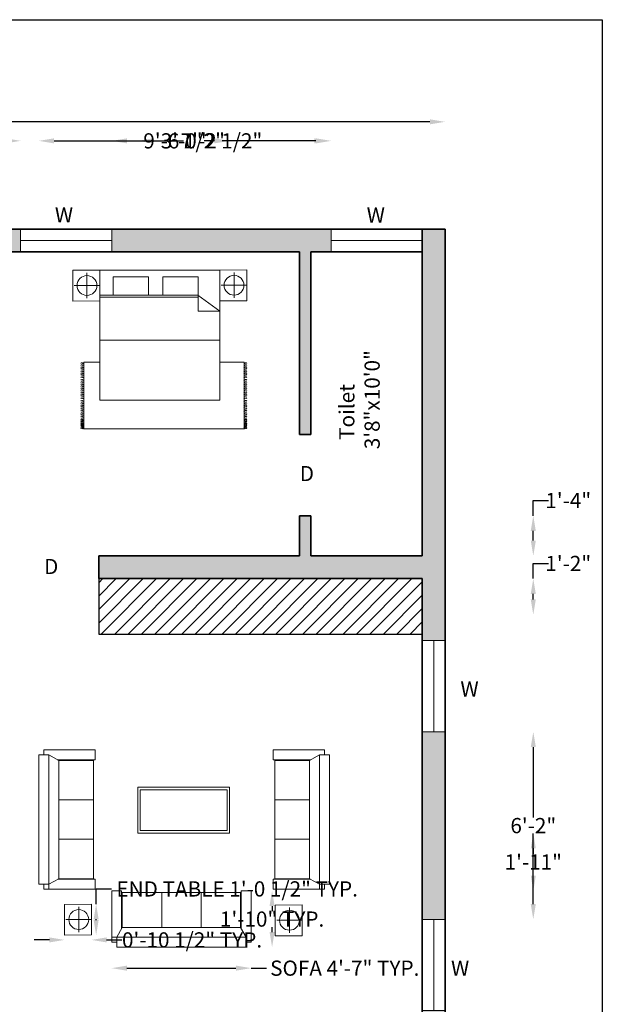
# Model space of a CAD drawing. Units: inches. Extents: x 1054 to 1577, y 4847 to 5610.
# Tile 5 of 5: x 1347 to 1577, y 5221 to 5610. Entities that reach past the tile are written whole.
import ezdxf

# ---------------------------------------------------------------- set-up
doc = ezdxf.new("R2010")
doc.units = ezdxf.units.IN
doc.header["$MEASUREMENT"] = 0
for name, color, linetype, lineweight in [('A-ANNO-DIMS', 2, 'Continuous', 18), ('A-ANNO-TEXT', 7, 'Continuous', 18), ('A-ANNO-TTLB', 7, 'Continuous', 25), ('A-AREA-IDEN', 7, 'Continuous', 18), ('A-FLOR-CASE', 7, 'Continuous', 25), ('A-FLOR-CASE-PATT', 252, 'Continuous', 13), ('A-GLAZ', 4, 'Continuous', 18), ('A-WALL', 7, 'Continuous', 35)]:
    doc.layers.add(name, color=color, linetype=linetype, lineweight=lineweight)
doc.layers.add('A-FURN', color=40, linetype='Continuous', lineweight=18, true_color=0xf8d731)
doc.layers.add('A-WALL-PATT', color=240, linetype='Continuous', lineweight=13, true_color=0xed1f24)
doc.styles.get("Standard").update_dxf_attribs({"font": 'arial.ttf'})
doc.dimstyles.get("Standard").update_dxf_attribs({"dimtxt": 6, "dimasz": 6, "dimexe": 0.18, "dimexo": 0.0625, "dimgap": 0.09, "dimtad": 0, "dimtih": 1, "dimtoh": 1, "dimdec": 1, "dimzin": 0, "dimdsep": 46, "dimlunit": 3, "dimtxsty": 'Standard', "dimcen": 0.09, "dimse1": 1, "dimse2": 1, "dimadec": 0, "dimazin": 0, "dimtfac": 1, "dimtdec": 1, "dimtofl": 0, "dimtmove": 0, "dimatfit": 3, "dimfxl": 1, "dimtolj": 1, "dimtzin": 0, "dimarcsym": 0})

# ---------------------------------------------------------------- blocks, each defined once
blk = doc.blocks.new('*D4')
at = {"layer": 'A-ANNO-DIMS', "color": 0, "lineweight": -2, "transparency": 16777216}
for p, q in [((1136.77, 5569.79), (1309.14, 5569.79)), ((1509.27, 5569.79), (1336.91, 5569.79))]:
    blk.add_line(p, q, dxfattribs=at)
at = {"layer": 'A-ANNO-DIMS', "color": 0, "transparency": 16777216}
for points in [[(1136.77, 5570.79), (1136.77, 5568.79), (1130.77, 5569.79)], [(1509.27, 5570.79), (1509.27, 5568.79), (1515.27, 5569.79)]]:
    blk.add_solid(points, dxfattribs=at)
at = {"layer": 'Defpoints', "color": 0, "transparency": 16777216}
for p in [(1515.27, 5569.79), (1130.77, 5527.48), (1515.27, 5527.48)]:
    blk.add_point(p, dxfattribs=at)
at = {"layer": 'A-ANNO-DIMS', "color": 0, "transparency": 16777216, "insert": (1323.02, 5569.79), "char_height": 6, "attachment_point": 5}
blk.add_mtext('\\A1;32\'-0.5"', dxfattribs=at)
blk = doc.blocks.new('WINDOW-36IN')
for p, q in [((0, 9), (0, 0)), ((36, 9), (0, 9)), ((36, 0), (36, 9)), ((36, 4.5), (0, 4.5)), ((0, 0), (36, 0))]:
    blk.add_line(p, q)
blk = doc.blocks.new('BED-DOUBLE-WITH-TABLES')
for p, q in [((5.6, 61.62), (5.6, 51.56)), ((63.65, 61.72), (63.65, 51.66)), ((10.63, 56.59), (0.57, 56.59)), ((68.68, 56.69), (58.62, 56.69)), ((49.39, 52.82), (10.63, 52.82)), ((49.44, 52), (10.63, 52)), ((49.39, 52.82), (58, 46.47)), ((49.44, 52.82), (49.44, 46.47)), ((49.44, 46.47), (58, 46.47)), ((58.05, 34.96), (10.63, 34.96)), ((4.35, 0), (4.35, 26.37)), ((4.35, 26.37), (10.65, 26.37)), ((58.05, 26.37), (67.59, 26.37)), ((67.59, 26.37), (67.59, 0)), ((67.59, 0), (4.35, 0))]:
    blk.add_line(p, q)
for points in [[(0, 50.39), (10.63, 50.5), (10.63, 62.68), (0, 62.58)], [(58.05, 62.68), (58.05, 11.37), (10.63, 11.37), (10.63, 62.68)], [(58.05, 50.5), (68.68, 50.6), (68.68, 62.78), (58.05, 62.68)], [(29.88, 59.98), (29.88, 52.82), (15.98, 52.82), (15.98, 59.98)], [(49.44, 59.98), (49.44, 52.82), (35.55, 52.82), (35.55, 59.98)]]:
    blk.add_lwpolyline(points, close=True)
for centre in [(5.6, 56.59), (63.65, 56.69)]:
    blk.add_circle(centre, 3.92)
for points, knots in [([(3.23, 25.84), (3.32, 25.96), (3.52, 26.2), (3.86, 25.96), (4.14, 25.78), (4.29, 25.89), (4.35, 25.94)], [0, 0, 0, 0, 0.400747, 0.791423, 1.067667, 1.29709, 1.29709, 1.29709, 1.29709]), ([(3.23, 25.06), (3.32, 25.18), (3.52, 25.42), (3.86, 25.18), (4.14, 25.01), (4.29, 25.11), (4.35, 25.16)], [0, 0, 0, 0, 0.400747, 0.791423, 1.067667, 1.29709, 1.29709, 1.29709, 1.29709]), ([(3.23, 24.24), (3.32, 24.36), (3.52, 24.6), (3.86, 24.36), (4.14, 24.19), (4.29, 24.3), (4.35, 24.34)], [0, 0, 0, 0, 0.400747, 0.791423, 1.067667, 1.29709, 1.29709, 1.29709, 1.29709]), ([(3.23, 23.51), (3.32, 23.63), (3.52, 23.87), (3.86, 23.63), (4.14, 23.46), (4.29, 23.57), (4.35, 23.62)], [0, 0, 0, 0, 0.400747, 0.791423, 1.067667, 1.29709, 1.29709, 1.29709, 1.29709]), ([(68.71, 25.84), (68.61, 25.96), (68.42, 26.2), (68.08, 25.96), (67.8, 25.78), (67.65, 25.89), (67.58, 25.94)], [0, 0, 0, 0, 0.400747, 0.791423, 1.067667, 1.29709, 1.29709, 1.29709, 1.29709]), ([(68.71, 25.06), (68.61, 25.18), (68.42, 25.42), (68.08, 25.18), (67.8, 25.01), (67.65, 25.11), (67.58, 25.16)], [0, 0, 0, 0, 0.400747, 0.791423, 1.067667, 1.29709, 1.29709, 1.29709, 1.29709]), ([(68.71, 24.24), (68.61, 24.36), (68.42, 24.6), (68.08, 24.36), (67.8, 24.19), (67.65, 24.3), (67.58, 24.34)], [0, 0, 0, 0, 0.400747, 0.791423, 1.067667, 1.29709, 1.29709, 1.29709, 1.29709]), ([(68.71, 23.51), (68.61, 23.63), (68.42, 23.87), (68.08, 23.63), (67.8, 23.46), (67.65, 23.57), (67.58, 23.62)], [0, 0, 0, 0, 0.400747, 0.791423, 1.067667, 1.29709, 1.29709, 1.29709, 1.29709]), ([(3.23, 22.63), (3.32, 22.75), (3.52, 22.99), (3.86, 22.75), (4.14, 22.58), (4.29, 22.69), (4.35, 22.73)], [0, 0, 0, 0, 0.400747, 0.791423, 1.067667, 1.29709, 1.29709, 1.29709, 1.29709]), ([(3.23, 21.88), (3.32, 22), (3.52, 22.24), (3.86, 22), (4.14, 21.83), (4.29, 21.93), (4.35, 21.98)], [0, 0, 0, 0, 0.400747, 0.791423, 1.067667, 1.29709, 1.29709, 1.29709, 1.29709]), ([(3.23, 21.15), (3.32, 21.27), (3.52, 21.51), (3.86, 21.27), (4.14, 21.1), (4.29, 21.21), (4.35, 21.25)], [0, 0, 0, 0, 0.400747, 0.791423, 1.067667, 1.29709, 1.29709, 1.29709, 1.29709]), ([(3.23, 20.27), (3.32, 20.39), (3.52, 20.63), (3.86, 20.39), (4.14, 20.22), (4.29, 20.32), (4.35, 20.37)], [0, 0, 0, 0, 0.400747, 0.791423, 1.067667, 1.29709, 1.29709, 1.29709, 1.29709]), ([(3.23, 19.23), (3.32, 19.35), (3.52, 19.59), (3.86, 19.35), (4.14, 19.18), (4.29, 19.29), (4.35, 19.33)], [0, 0, 0, 0, 0.400747, 0.791423, 1.067667, 1.29709, 1.29709, 1.29709, 1.29709]), ([(68.71, 22.63), (68.61, 22.75), (68.42, 22.99), (68.08, 22.75), (67.8, 22.58), (67.65, 22.69), (67.58, 22.73)], [0, 0, 0, 0, 0.400747, 0.791423, 1.067667, 1.29709, 1.29709, 1.29709, 1.29709]), ([(68.71, 21.88), (68.61, 22), (68.42, 22.24), (68.08, 22), (67.8, 21.83), (67.65, 21.93), (67.58, 21.98)], [0, 0, 0, 0, 0.400747, 0.791423, 1.067667, 1.29709, 1.29709, 1.29709, 1.29709]), ([(68.71, 21.15), (68.61, 21.27), (68.42, 21.51), (68.08, 21.27), (67.8, 21.1), (67.65, 21.21), (67.58, 21.25)], [0, 0, 0, 0, 0.400747, 0.791423, 1.067667, 1.29709, 1.29709, 1.29709, 1.29709]), ([(68.71, 20.27), (68.61, 20.39), (68.42, 20.63), (68.08, 20.39), (67.8, 20.22), (67.65, 20.32), (67.58, 20.37)], [0, 0, 0, 0, 0.400747, 0.791423, 1.067667, 1.29709, 1.29709, 1.29709, 1.29709]), ([(68.71, 19.23), (68.61, 19.35), (68.42, 19.59), (68.08, 19.35), (67.8, 19.18), (67.65, 19.29), (67.58, 19.33)], [0, 0, 0, 0, 0.400747, 0.791423, 1.067667, 1.29709, 1.29709, 1.29709, 1.29709]), ([(3.23, 18.35), (3.32, 18.47), (3.52, 18.71), (3.86, 18.47), (4.14, 18.3), (4.29, 18.4), (4.35, 18.45)], [0, 0, 0, 0, 0.400747, 0.791423, 1.067667, 1.29709, 1.29709, 1.29709, 1.29709]), ([(3.23, 17.53), (3.32, 17.65), (3.52, 17.89), (3.86, 17.65), (4.14, 17.48), (4.29, 17.59), (4.35, 17.64)], [0, 0, 0, 0, 0.400747, 0.791423, 1.067667, 1.29709, 1.29709, 1.29709, 1.29709]), ([(3.23, 16.76), (3.32, 16.88), (3.52, 17.12), (3.86, 16.88), (4.14, 16.71), (4.29, 16.81), (4.35, 16.86)], [0, 0, 0, 0, 0.400747, 0.791423, 1.067667, 1.29709, 1.29709, 1.29709, 1.29709]), ([(3.23, 15.94), (3.32, 16.06), (3.52, 16.3), (3.86, 16.06), (4.14, 15.89), (4.29, 16), (4.35, 16.04)], [0, 0, 0, 0, 0.400747, 0.791423, 1.067667, 1.29709, 1.29709, 1.29709, 1.29709]), ([(68.71, 18.35), (68.61, 18.47), (68.42, 18.71), (68.08, 18.47), (67.8, 18.3), (67.65, 18.4), (67.58, 18.45)], [0, 0, 0, 0, 0.400747, 0.791423, 1.067667, 1.29709, 1.29709, 1.29709, 1.29709]), ([(68.71, 17.53), (68.61, 17.65), (68.42, 17.89), (68.08, 17.65), (67.8, 17.48), (67.65, 17.59), (67.58, 17.64)], [0, 0, 0, 0, 0.400747, 0.791423, 1.067667, 1.29709, 1.29709, 1.29709, 1.29709]), ([(68.71, 16.76), (68.61, 16.88), (68.42, 17.12), (68.08, 16.88), (67.8, 16.71), (67.65, 16.81), (67.58, 16.86)], [0, 0, 0, 0, 0.400747, 0.791423, 1.067667, 1.29709, 1.29709, 1.29709, 1.29709]), ([(68.71, 15.94), (68.61, 16.06), (68.42, 16.3), (68.08, 16.06), (67.8, 15.89), (67.65, 16), (67.58, 16.04)], [0, 0, 0, 0, 0.400747, 0.791423, 1.067667, 1.29709, 1.29709, 1.29709, 1.29709]), ([(3.23, 15.21), (3.32, 15.33), (3.52, 15.57), (3.86, 15.33), (4.14, 15.16), (4.29, 15.27), (4.35, 15.32)], [0, 0, 0, 0, 0.400747, 0.791423, 1.067667, 1.29709, 1.29709, 1.29709, 1.29709]), ([(3.23, 14.33), (3.32, 14.45), (3.52, 14.69), (3.86, 14.45), (4.14, 14.28), (4.29, 14.39), (4.35, 14.43)], [0, 0, 0, 0, 0.400747, 0.791423, 1.067667, 1.29709, 1.29709, 1.29709, 1.29709]), ([(3.23, 13.58), (3.32, 13.7), (3.52, 13.94), (3.86, 13.7), (4.14, 13.53), (4.29, 13.63), (4.35, 13.68)], [0, 0, 0, 0, 0.400747, 0.791423, 1.067667, 1.29709, 1.29709, 1.29709, 1.29709]), ([(3.23, 12.85), (3.32, 12.97), (3.52, 13.21), (3.86, 12.97), (4.14, 12.8), (4.29, 12.9), (4.35, 12.95)], [0, 0, 0, 0, 0.400747, 0.791423, 1.067667, 1.29709, 1.29709, 1.29709, 1.29709]), ([(3.23, 11.97), (3.32, 12.09), (3.52, 12.33), (3.86, 12.09), (4.14, 11.92), (4.29, 12.02), (4.35, 12.07)], [0, 0, 0, 0, 0.400747, 0.791423, 1.067667, 1.29709, 1.29709, 1.29709, 1.29709]), ([(68.71, 15.21), (68.61, 15.33), (68.42, 15.57), (68.08, 15.33), (67.8, 15.16), (67.65, 15.27), (67.58, 15.32)], [0, 0, 0, 0, 0.400747, 0.791423, 1.067667, 1.29709, 1.29709, 1.29709, 1.29709]), ([(68.71, 14.33), (68.61, 14.45), (68.42, 14.69), (68.08, 14.45), (67.8, 14.28), (67.65, 14.39), (67.58, 14.43)], [0, 0, 0, 0, 0.400747, 0.791423, 1.067667, 1.29709, 1.29709, 1.29709, 1.29709]), ([(68.71, 13.58), (68.61, 13.7), (68.42, 13.94), (68.08, 13.7), (67.8, 13.53), (67.65, 13.63), (67.58, 13.68)], [0, 0, 0, 0, 0.400747, 0.791423, 1.067667, 1.29709, 1.29709, 1.29709, 1.29709]), ([(68.71, 12.85), (68.61, 12.97), (68.42, 13.21), (68.08, 12.97), (67.8, 12.8), (67.65, 12.9), (67.58, 12.95)], [0, 0, 0, 0, 0.400747, 0.791423, 1.067667, 1.29709, 1.29709, 1.29709, 1.29709]), ([(68.71, 11.97), (68.61, 12.09), (68.42, 12.33), (68.08, 12.09), (67.8, 11.92), (67.65, 12.02), (67.58, 12.07)], [0, 0, 0, 0, 0.400747, 0.791423, 1.067667, 1.29709, 1.29709, 1.29709, 1.29709]), ([(3.23, 10.93), (3.32, 11.05), (3.52, 11.29), (3.86, 11.05), (4.14, 10.88), (4.29, 10.99), (4.35, 11.03)], [0, 0, 0, 0, 0.400747, 0.791423, 1.067667, 1.29709, 1.29709, 1.29709, 1.29709]), ([(3.23, 10.05), (3.32, 10.17), (3.52, 10.41), (3.86, 10.17), (4.14, 10), (4.29, 10.1), (4.35, 10.15)], [0, 0, 0, 0, 0.400747, 0.791423, 1.067667, 1.29709, 1.29709, 1.29709, 1.29709]), ([(3.23, 9.23), (3.32, 9.35), (3.52, 9.59), (3.86, 9.35), (4.14, 9.18), (4.29, 9.29), (4.35, 9.34)], [0, 0, 0, 0, 0.400747, 0.791423, 1.067667, 1.29709, 1.29709, 1.29709, 1.29709]), ([(3.23, 8.54), (3.32, 8.66), (3.52, 8.9), (3.86, 8.66), (4.14, 8.49), (4.29, 8.6), (4.35, 8.65)], [0, 0, 0, 0, 0.400747, 0.791423, 1.067667, 1.29709, 1.29709, 1.29709, 1.29709]), ([(3.23, 7.73), (3.32, 7.85), (3.52, 8.09), (3.86, 7.85), (4.14, 7.68), (4.29, 7.78), (4.35, 7.83)], [0, 0, 0, 0, 0.400747, 0.791423, 1.067667, 1.29709, 1.29709, 1.29709, 1.29709]), ([(68.71, 10.93), (68.61, 11.05), (68.42, 11.29), (68.08, 11.05), (67.8, 10.88), (67.65, 10.99), (67.58, 11.03)], [0, 0, 0, 0, 0.400747, 0.791423, 1.067667, 1.29709, 1.29709, 1.29709, 1.29709]), ([(68.71, 10.05), (68.61, 10.17), (68.42, 10.41), (68.08, 10.17), (67.8, 10), (67.65, 10.1), (67.58, 10.15)], [0, 0, 0, 0, 0.400747, 0.791423, 1.067667, 1.29709, 1.29709, 1.29709, 1.29709]), ([(68.71, 9.23), (68.61, 9.35), (68.42, 9.59), (68.08, 9.35), (67.8, 9.18), (67.65, 9.29), (67.58, 9.34)], [0, 0, 0, 0, 0.400747, 0.791423, 1.067667, 1.29709, 1.29709, 1.29709, 1.29709]), ([(68.71, 8.54), (68.61, 8.66), (68.42, 8.9), (68.08, 8.66), (67.8, 8.49), (67.65, 8.6), (67.58, 8.65)], [0, 0, 0, 0, 0.400747, 0.791423, 1.067667, 1.29709, 1.29709, 1.29709, 1.29709]), ([(68.71, 7.73), (68.61, 7.85), (68.42, 8.09), (68.08, 7.85), (67.8, 7.68), (67.65, 7.78), (67.58, 7.83)], [0, 0, 0, 0, 0.400747, 0.791423, 1.067667, 1.29709, 1.29709, 1.29709, 1.29709]), ([(3.23, 7), (3.32, 7.12), (3.52, 7.36), (3.86, 7.12), (4.14, 6.95), (4.29, 7.05), (4.35, 7.1)], [0, 0, 0, 0, 0.400747, 0.791423, 1.067667, 1.29709, 1.29709, 1.29709, 1.29709]), ([(3.23, 6.12), (3.32, 6.24), (3.52, 6.48), (3.86, 6.24), (4.14, 6.07), (4.29, 6.17), (4.35, 6.22)], [0, 0, 0, 0, 0.400747, 0.791423, 1.067667, 1.29709, 1.29709, 1.29709, 1.29709]), ([(3.23, 5.36), (3.32, 5.49), (3.52, 5.73), (3.86, 5.49), (4.14, 5.31), (4.29, 5.42), (4.35, 5.47)], [0, 0, 0, 0, 0.400747, 0.791423, 1.067667, 1.29709, 1.29709, 1.29709, 1.29709]), ([(3.23, 4.64), (3.32, 4.76), (3.52, 5), (3.86, 4.76), (4.14, 4.59), (4.29, 4.69), (4.35, 4.74)], [0, 0, 0, 0, 0.400747, 0.791423, 1.067667, 1.29709, 1.29709, 1.29709, 1.29709]), ([(3.23, 3.75), (3.32, 3.88), (3.52, 4.12), (3.86, 3.88), (4.14, 3.7), (4.29, 3.81), (4.35, 3.86)], [0, 0, 0, 0, 0.400747, 0.791423, 1.067667, 1.29709, 1.29709, 1.29709, 1.29709]), ([(68.71, 7), (68.61, 7.12), (68.42, 7.36), (68.08, 7.12), (67.8, 6.95), (67.65, 7.05), (67.58, 7.1)], [0, 0, 0, 0, 0.400747, 0.791423, 1.067667, 1.29709, 1.29709, 1.29709, 1.29709]), ([(68.71, 6.12), (68.61, 6.24), (68.42, 6.48), (68.08, 6.24), (67.8, 6.07), (67.65, 6.17), (67.58, 6.22)], [0, 0, 0, 0, 0.400747, 0.791423, 1.067667, 1.29709, 1.29709, 1.29709, 1.29709]), ([(68.71, 5.36), (68.61, 5.49), (68.42, 5.73), (68.08, 5.49), (67.8, 5.31), (67.65, 5.42), (67.58, 5.47)], [0, 0, 0, 0, 0.400747, 0.791423, 1.067667, 1.29709, 1.29709, 1.29709, 1.29709]), ([(68.71, 4.64), (68.61, 4.76), (68.42, 5), (68.08, 4.76), (67.8, 4.59), (67.66, 4.69), (67.59, 4.73)], [0, 0, 0, 0, 0.400747, 0.791423, 1.067667, 1.283686, 1.283686, 1.283686, 1.283686]), ([(68.71, 3.75), (68.61, 3.88), (68.42, 4.12), (68.08, 3.88), (67.8, 3.7), (67.66, 3.81), (67.59, 3.85)], [0, 0, 0, 0, 0.400747, 0.791423, 1.067667, 1.283686, 1.283686, 1.283686, 1.283686]), ([(3.23, 3.33), (3.32, 3.45), (3.51, 3.7), (3.86, 3.44), (4.14, 3.27), (4.29, 3.38), (4.35, 3.43)], [0, 0, 0, 0, 0.407265, 0.802015, 1.07826, 1.307683, 1.307683, 1.307683, 1.307683]), ([(3.23, 2.76), (3.32, 2.88), (3.52, 3.12), (3.86, 2.88), (4.14, 2.71), (4.29, 2.81), (4.35, 2.86)], [0, 0, 0, 0, 0.400747, 0.791423, 1.067667, 1.29709, 1.29709, 1.29709, 1.29709]), ([(3.23, 2.19), (3.32, 2.31), (3.52, 2.55), (3.86, 2.31), (4.14, 2.13), (4.29, 2.24), (4.35, 2.29)], [0, 0, 0, 0, 0.400747, 0.791423, 1.067667, 1.29709, 1.29709, 1.29709, 1.29709]), ([(3.23, 1.88), (3.32, 2), (3.52, 2.24), (3.86, 2), (4.14, 1.82), (4.29, 1.93), (4.35, 1.98)], [0, 0, 0, 0, 0.400747, 0.791423, 1.067667, 1.29709, 1.29709, 1.29709, 1.29709]), ([(3.23, 1.46), (3.32, 1.58), (3.52, 1.82), (3.86, 1.58), (4.14, 1.41), (4.29, 1.51), (4.35, 1.56)], [0, 0, 0, 0, 0.400747, 0.791423, 1.067667, 1.29709, 1.29709, 1.29709, 1.29709]), ([(3.23, 1.06), (3.32, 1.18), (3.52, 1.42), (3.86, 1.18), (4.14, 1.01), (4.29, 1.11), (4.35, 1.16)], [0, 0, 0, 0, 0.400747, 0.791423, 1.067667, 1.29709, 1.29709, 1.29709, 1.29709]), ([(3.23, 0.57), (3.32, 0.7), (3.52, 0.94), (3.86, 0.7), (4.14, 0.52), (4.29, 0.63), (4.35, 0.68)], [0, 0, 0, 0, 0.400747, 0.791423, 1.067667, 1.29709, 1.29709, 1.29709, 1.29709]), ([(3.23, 0.07), (3.32, 0.19), (3.52, 0.43), (3.86, 0.19), (4.14, 0.02), (4.29, 0.13), (4.35, 0.18)], [0, 0, 0, 0, 0.400747, 0.791423, 1.067667, 1.29709, 1.29709, 1.29709, 1.29709]), ([(68.71, 1.43), (68.61, 1.55), (68.42, 1.79), (68.08, 1.55), (67.8, 1.38), (67.65, 1.48), (67.58, 1.53)], [0, 0, 0, 0, 0.400747, 0.791423, 1.067667, 1.29709, 1.29709, 1.29709, 1.29709]), ([(68.71, 1.03), (68.61, 1.15), (68.42, 1.39), (68.08, 1.15), (67.8, 0.98), (67.65, 1.09), (67.58, 1.13)], [0, 0, 0, 0, 0.400747, 0.791423, 1.067667, 1.29709, 1.29709, 1.29709, 1.29709]), ([(68.71, 0.55), (68.61, 0.67), (68.42, 0.91), (68.08, 0.67), (67.8, 0.5), (67.65, 0.6), (67.58, 0.65)], [0, 0, 0, 0, 0.400747, 0.791423, 1.067667, 1.29709, 1.29709, 1.29709, 1.29709]), ([(68.71, 0.07), (68.61, 0.19), (68.42, 0.43), (68.08, 0.19), (67.8, 0.02), (67.65, 0.13), (67.58, 0.18)], [0, 0, 0, 0, 0.400747, 0.791423, 1.067667, 1.29709, 1.29709, 1.29709, 1.29709]), ([(68.71, 3.33), (68.61, 3.45), (68.42, 3.69), (68.08, 3.45), (67.8, 3.28), (67.66, 3.38), (67.59, 3.42)], [0, 0, 0, 0, 0.402903, 0.794912, 1.071156, 1.287177, 1.287177, 1.287177, 1.287177]), ([(68.71, 2.73), (68.61, 2.85), (68.42, 3.09), (68.08, 2.85), (67.8, 2.68), (67.66, 2.78), (67.59, 2.83)], [0, 0, 0, 0, 0.400747, 0.791423, 1.067667, 1.283686, 1.283686, 1.283686, 1.283686]), ([(68.71, 2.16), (68.61, 2.28), (68.42, 2.52), (68.08, 2.28), (67.8, 2.11), (67.66, 2.21), (67.59, 2.25)], [0, 0, 0, 0, 0.400747, 0.791423, 1.067667, 1.283686, 1.283686, 1.283686, 1.283686]), ([(68.71, 1.85), (68.61, 1.97), (68.42, 2.21), (68.08, 1.97), (67.8, 1.8), (67.66, 1.9), (67.59, 1.94)], [0, 0, 0, 0, 0.400747, 0.791423, 1.067667, 1.283686, 1.283686, 1.283686, 1.283686])]:
    blk.add_open_spline(points, degree=3, knots=knots)
blk = doc.blocks.new('SOFA-3SEAT')
for p, q in [((0, 1.96), (0, 22.23)), ((3.92, 22.23), (0, 22.23)), ((3.92, 7.54), (3.92, 22.23)), ((4.17, 21.58), (4.17, 7.85)), ((19.74, 21.58), (19.74, 7.85)), ((35.31, 21.58), (35.31, 7.85)), ((51.12, 7.29), (51.12, 22.23)), ((51.12, 22.23), (55.04, 22.23)), ((55.04, 1.96), (55.04, 22.23)), ((1.96, 3.92), (4.17, 7.85)), ((50.88, 7.85), (53.08, 3.92)), ((0, 3.92), (53.08, 3.92)), ((1.96, 3.92), (1.96, 0)), ((53.08, 3.92), (53.08, 0)), ((0, 1.96), (1.96, 1.96)), ((1.96, 0), (53.08, 0)), ((53.08, 1.96), (55.04, 1.96))]:
    blk.add_line(p, q)
blk.add_lwpolyline([(4.17, 7.85), (50.88, 7.85), (50.88, 21.58), (4.17, 21.58)])
blk = doc.blocks.new('END-TABLE-PLAN')
for p, q in [((5.6, 11.22), (5.6, 1.17)), ((10.63, 6.2), (0.57, 6.2))]:
    blk.add_line(p, q)
blk.add_lwpolyline([(0, 0), (10.63, 0.1), (10.63, 12.29), (0, 12.19)], close=True)
blk.add_circle((5.6, 6.2), 3.92)
blk = doc.blocks.new('*D14')
at = {"layer": 'A-ANNO-DIMS', "color": 0, "lineweight": -2, "transparency": 16777216}
for p, q in [((1389.68, 5235.75), (1432.73, 5235.75)), ((1438.73, 5235.75), (1444.73, 5235.75))]:
    blk.add_line(p, q, dxfattribs=at)
at = {"layer": 'A-ANNO-DIMS', "color": 0, "transparency": 16777216}
for points in [[(1389.68, 5236.75), (1389.68, 5234.75), (1383.68, 5235.75)], [(1432.73, 5236.75), (1432.73, 5234.75), (1438.73, 5235.75)]]:
    blk.add_solid(points, dxfattribs=at)
at = {"layer": 'Defpoints', "color": 0, "transparency": 16777216}
for p in [(1383.68, 5244.01), (1438.73, 5244.01), (1438.73, 5235.75)]:
    blk.add_point(p, dxfattribs=at)
at = {"layer": 'A-ANNO-DIMS', "color": 0, "transparency": 16777216, "insert": (1475.66, 5235.75), "char_height": 6, "attachment_point": 5}
blk.add_mtext('\\A1;SOFA 4\'-7" TYP.', dxfattribs=at)
blk = doc.blocks.new('*D15')
at = {"layer": 'A-ANNO-DIMS', "color": 0, "lineweight": -2, "transparency": 16777216}
for p, q in [((1446.98, 5260.24), (1446.98, 5258.28)), ((1446.98, 5250.01), (1446.98, 5251.97))]:
    blk.add_line(p, q, dxfattribs=at)
at = {"layer": 'A-ANNO-DIMS', "color": 0, "transparency": 16777216}
for points in [[(1445.98, 5260.24), (1447.98, 5260.24), (1446.98, 5266.24)], [(1445.98, 5250.01), (1447.98, 5250.01), (1446.98, 5244.01)]]:
    blk.add_solid(points, dxfattribs=at)
at = {"layer": 'Defpoints', "color": 0, "transparency": 16777216}
for p in [(1438.73, 5266.24), (1446.98, 5266.24), (1438.73, 5244.01)]:
    blk.add_point(p, dxfattribs=at)
at = {"layer": 'A-ANNO-DIMS', "color": 0, "transparency": 16777216, "insert": (1446.98, 5255.12), "char_height": 6, "attachment_point": 5}
blk.add_mtext('\\A1;1\'-10" TYP.', dxfattribs=at)
blk = doc.blocks.new('*D16')
at = {"layer": 'A-ANNO-DIMS', "color": 0, "lineweight": -2, "transparency": 16777216}
for p, q in [((1377.54, 5261.03), (1377.54, 5267.03)), ((1377.54, 5267.03), (1383.54, 5267.03)), ((1377.54, 5254.74), (1377.54, 5255.03))]:
    blk.add_line(p, q, dxfattribs=at)
at = {"layer": 'A-ANNO-DIMS', "color": 0, "transparency": 16777216}
for points in [[(1376.54, 5255.03), (1378.54, 5255.03), (1377.54, 5261.03)], [(1376.54, 5254.74), (1378.54, 5254.74), (1377.54, 5248.74)]]:
    blk.add_solid(points, dxfattribs=at)
at = {"layer": 'Defpoints', "color": 0, "transparency": 16777216}
for p in [(1375.69, 5261.03), (1377.54, 5261.03), (1375.69, 5248.74)]:
    blk.add_point(p, dxfattribs=at)
at = {"layer": 'A-ANNO-DIMS', "color": 0, "transparency": 16777216, "insert": (1433.2, 5267.03), "char_height": 6, "attachment_point": 5}
blk.add_mtext('\\A1;END TABLE 1\'-0 1/2" TYP.', dxfattribs=at)
blk = doc.blocks.new('*D17')
at = {"layer": 'A-ANNO-DIMS', "color": 0, "lineweight": -2, "transparency": 16777216}
for p, q in [((1359.07, 5246.9), (1353.07, 5246.9)), ((1381.69, 5246.9), (1387.69, 5246.9))]:
    blk.add_line(p, q, dxfattribs=at)
at = {"layer": 'A-ANNO-DIMS', "color": 0, "transparency": 16777216}
for points in [[(1359.07, 5247.9), (1359.07, 5245.9), (1365.07, 5246.9)], [(1381.69, 5247.9), (1381.69, 5245.9), (1375.69, 5246.9)]]:
    blk.add_solid(points, dxfattribs=at)
at = {"layer": 'Defpoints', "color": 0, "transparency": 16777216}
for p in [(1365.07, 5248.74), (1375.69, 5248.74), (1375.69, 5246.9)]:
    blk.add_point(p, dxfattribs=at)
at = {"layer": 'A-ANNO-DIMS', "color": 0, "transparency": 16777216, "insert": (1415.39, 5246.9), "char_height": 6, "attachment_point": 5}
blk.add_mtext('\\A1;0\'-10 1/2" TYP.', dxfattribs=at)
blk = doc.blocks.new('*D25')
at = {"layer": 'A-ANNO-DIMS', "color": 0, "lineweight": -2, "transparency": 16777216}
for p, q in [((1348.59, 4855.83), (1352.52, 4855.83)), ((1372.59, 4855.83), (1368.65, 4855.83))]:
    blk.add_line(p, q, dxfattribs=at)
at = {"layer": 'A-ANNO-DIMS', "color": 0, "transparency": 16777216}
for points in [[(1348.59, 4856.83), (1348.59, 4854.83), (1342.59, 4855.83)], [(1372.59, 4856.83), (1372.59, 4854.83), (1378.59, 4855.83)]]:
    blk.add_solid(points, dxfattribs=at)
at = {"layer": 'Defpoints', "color": 0, "transparency": 16777216}
for p in [(1342.59, 5389.48), (1378.59, 5389.48), (1378.59, 4855.83)]:
    blk.add_point(p, dxfattribs=at)
at = {"layer": 'A-ANNO-DIMS', "color": 0, "transparency": 16777216, "insert": (1360.59, 4855.83), "char_height": 6, "attachment_point": 5}
blk.add_mtext('\\A1;3\'-0"', dxfattribs=at)
blk = doc.blocks.new('*D30')
at = {"layer": 'A-ANNO-DIMS', "color": 0, "lineweight": -2, "transparency": 16777216}
for p, q in [((1255.08, 5562.28), (1283.35, 5562.28)), ((1341.75, 5562.28), (1313.47, 5562.28))]:
    blk.add_line(p, q, dxfattribs=at)
at = {"layer": 'A-ANNO-DIMS', "color": 0, "transparency": 16777216}
for points in [[(1255.08, 5563.28), (1255.08, 5561.28), (1249.08, 5562.28)], [(1341.75, 5563.28), (1341.75, 5561.28), (1347.75, 5562.28)]]:
    blk.add_solid(points, dxfattribs=at)
at = {"layer": 'Defpoints', "color": 0, "transparency": 16777216}
for p in [(1347.75, 5562.28), (1249.08, 5527.48), (1347.75, 5527.48)]:
    blk.add_point(p, dxfattribs=at)
at = {"layer": 'A-ANNO-DIMS', "color": 0, "transparency": 16777216, "insert": (1298.41, 5562.28), "char_height": 6, "attachment_point": 5}
blk.add_mtext('\\A1;8\'-2 1/2"', dxfattribs=at)
blk = doc.blocks.new('*D31')
at = {"layer": 'A-ANNO-DIMS', "color": 0, "lineweight": -2, "transparency": 16777216}
for p, q in [((1389.75, 5562.28), (1411.98, 5562.28)), ((1464.27, 5562.28), (1442.04, 5562.28))]:
    blk.add_line(p, q, dxfattribs=at)
at = {"layer": 'A-ANNO-DIMS', "color": 0, "transparency": 16777216}
for points in [[(1389.75, 5563.28), (1389.75, 5561.28), (1383.75, 5562.28)], [(1464.27, 5563.28), (1464.27, 5561.28), (1470.27, 5562.28)]]:
    blk.add_solid(points, dxfattribs=at)
at = {"layer": 'Defpoints', "color": 0, "transparency": 16777216}
for p in [(1470.27, 5562.28), (1383.75, 5527.48), (1470.27, 5527.48)]:
    blk.add_point(p, dxfattribs=at)
at = {"layer": 'A-ANNO-DIMS', "color": 0, "transparency": 16777216, "insert": (1427.01, 5562.28), "char_height": 6, "attachment_point": 5}
blk.add_mtext('\\A1;7\'-2 1/2"', dxfattribs=at)
blk = doc.blocks.new('*D36')
at = {"layer": 'A-ANNO-DIMS', "color": 0, "lineweight": -2, "transparency": 16777216}
for p, q in [((1550.07, 5323.03), (1550.07, 5295.17)), ((1550.07, 5261.01), (1550.07, 5288.87))]:
    blk.add_line(p, q, dxfattribs=at)
at = {"layer": 'A-ANNO-DIMS', "color": 0, "transparency": 16777216}
for points in [[(1549.07, 5323.03), (1551.07, 5323.03), (1550.07, 5329.03)], [(1549.07, 5261.01), (1551.07, 5261.01), (1550.07, 5255.01)]]:
    blk.add_solid(points, dxfattribs=at)
at = {"layer": 'Defpoints', "color": 0, "transparency": 16777216}
for p in [(1515.27, 5329.03), (1550.07, 5329.03), (1515.27, 5255.01)]:
    blk.add_point(p, dxfattribs=at)
at = {"layer": 'A-ANNO-DIMS', "color": 0, "transparency": 16777216, "insert": (1550.07, 5292.02), "char_height": 6, "attachment_point": 5}
blk.add_mtext('\\A1;6\'-2"', dxfattribs=at)
blk = doc.blocks.new('*D43')
at = {"layer": 'A-ANNO-DIMS', "color": 0, "lineweight": -2, "transparency": 16777216}
for p, q in [((1550.07, 5389.48), (1550.07, 5395.48)), ((1550.07, 5395.48), (1556.07, 5395.48)), ((1550.07, 5381.26), (1550.07, 5383.48))]:
    blk.add_line(p, q, dxfattribs=at)
at = {"layer": 'A-ANNO-DIMS', "color": 0, "transparency": 16777216}
for points in [[(1549.07, 5383.48), (1551.07, 5383.48), (1550.07, 5389.48)], [(1549.07, 5381.26), (1551.07, 5381.26), (1550.07, 5375.26)]]:
    blk.add_solid(points, dxfattribs=at)
at = {"layer": 'Defpoints', "color": 0, "transparency": 16777216}
for p in [(1268.77, 5389.48), (1550.07, 5389.48), (1268.77, 5375.26)]:
    blk.add_point(p, dxfattribs=at)
at = {"layer": 'A-ANNO-DIMS', "color": 0, "transparency": 16777216, "insert": (1563.86, 5395.48), "char_height": 6, "attachment_point": 5}
blk.add_mtext('\\A1;1\'-2"', dxfattribs=at)
blk = doc.blocks.new('*D45')
at = {"layer": 'A-ANNO-DIMS', "color": 0, "lineweight": -2, "transparency": 16777216}
for p, q in [((1550.07, 5414.33), (1550.07, 5420.33)), ((1550.07, 5420.33), (1556.07, 5420.33)), ((1550.07, 5404.48), (1550.07, 5408.33))]:
    blk.add_line(p, q, dxfattribs=at)
at = {"layer": 'A-ANNO-DIMS', "color": 0, "transparency": 16777216}
for points in [[(1549.07, 5408.33), (1551.07, 5408.33), (1550.07, 5414.33)], [(1549.07, 5404.48), (1551.07, 5404.48), (1550.07, 5398.48)]]:
    blk.add_solid(points, dxfattribs=at)
at = {"layer": 'Defpoints', "color": 0, "transparency": 16777216}
for p in [(1462.27, 5414.33), (1550.07, 5414.33), (1462.27, 5398.48)]:
    blk.add_point(p, dxfattribs=at)
at = {"layer": 'A-ANNO-DIMS', "color": 0, "transparency": 16777216, "insert": (1563.86, 5420.33), "char_height": 6, "attachment_point": 5}
blk.add_mtext('\\A1;1\'-4"', dxfattribs=at)
blk = doc.blocks.new('*D48')
at = {"layer": 'A-ANNO-DIMS', "color": 0, "lineweight": -2, "transparency": 16777216}
for p, q in [((1399.95, 5562.28), (1404.01, 5562.28)), ((1424.19, 5562.28), (1420.14, 5562.28))]:
    blk.add_line(p, q, dxfattribs=at)
at = {"layer": 'A-ANNO-DIMS', "color": 0, "transparency": 16777216}
for points in [[(1399.95, 5563.28), (1399.95, 5561.28), (1393.95, 5562.28)], [(1424.19, 5563.28), (1424.19, 5561.28), (1430.19, 5562.28)]]:
    blk.add_solid(points, dxfattribs=at)
at = {"layer": 'Defpoints', "color": 0, "transparency": 16777216}
for p in [(1430.19, 5562.28), (1393.95, 5307.18), (1430.19, 5307.18)]:
    blk.add_point(p, dxfattribs=at)
at = {"layer": 'A-ANNO-DIMS', "color": 0, "transparency": 16777216, "insert": (1412.07, 5562.28), "char_height": 6, "attachment_point": 5}
blk.add_mtext('\\A1;3\'-0"', dxfattribs=at)
blk = doc.blocks.new('*D49')
at = {"layer": 'A-ANNO-DIMS', "color": 0, "lineweight": -2, "transparency": 16777216}
for p, q in [((1095.97, 5307.18), (1095.97, 5313.18)), ((1095.97, 5313.18), (1101.97, 5313.18)), ((1095.97, 5295.07), (1095.97, 5301.18))]:
    blk.add_line(p, q, dxfattribs=at)
at = {"layer": 'A-ANNO-DIMS', "color": 0, "transparency": 16777216}
for points in [[(1094.97, 5301.18), (1096.97, 5301.18), (1095.97, 5307.18)], [(1094.97, 5295.07), (1096.97, 5295.07), (1095.97, 5289.07)]]:
    blk.add_solid(points, dxfattribs=at)
at = {"layer": 'Defpoints', "color": 0, "transparency": 16777216}
for p in [(1095.97, 5307.18), (1393.95, 5307.18), (1393.95, 5289.07)]:
    blk.add_point(p, dxfattribs=at)
at = {"layer": 'A-ANNO-DIMS', "color": 0, "transparency": 16777216, "insert": (1109.76, 5313.18), "char_height": 6, "attachment_point": 5}
blk.add_mtext('\\A1;1\'-6"', dxfattribs=at)
blk = doc.blocks.new('*D50')
at = {"layer": 'A-ANNO-DIMS', "color": 0, "lineweight": -2, "transparency": 16777216}
for p, q in [((1360.92, 5562.28), (1397.21, 5562.28)), ((1463.62, 5562.28), (1427.32, 5562.28))]:
    blk.add_line(p, q, dxfattribs=at)
at = {"layer": 'A-ANNO-DIMS', "color": 0, "transparency": 16777216}
for points in [[(1360.92, 5563.28), (1360.92, 5561.28), (1354.92, 5562.28)], [(1463.62, 5563.28), (1463.62, 5561.28), (1469.62, 5562.28)]]:
    blk.add_solid(points, dxfattribs=at)
at = {"layer": 'Defpoints', "color": 0, "transparency": 16777216}
for p in [(1469.62, 5562.28), (1354.92, 5319.98), (1469.62, 5319.98)]:
    blk.add_point(p, dxfattribs=at)
at = {"layer": 'A-ANNO-DIMS', "color": 0, "transparency": 16777216, "insert": (1412.27, 5562.28), "char_height": 6, "attachment_point": 5}
blk.add_mtext('\\A1;9\'-6 1/2"', dxfattribs=at)
blk = doc.blocks.new('*D51')
at = {"layer": 'A-ANNO-DIMS', "color": 0, "lineweight": -2, "transparency": 16777216}
for p, q in [((1095.97, 5315.94), (1095.97, 5286.13)), ((1095.97, 5250.01), (1095.97, 5279.82))]:
    blk.add_line(p, q, dxfattribs=at)
at = {"layer": 'A-ANNO-DIMS', "color": 0, "transparency": 16777216}
for points in [[(1094.97, 5315.94), (1096.97, 5315.94), (1095.97, 5321.94)], [(1094.97, 5250.01), (1096.97, 5250.01), (1095.97, 5244.01)]]:
    blk.add_solid(points, dxfattribs=at)
at = {"layer": 'Defpoints', "color": 0, "transparency": 16777216}
for p in [(1095.97, 5321.94), (1356.88, 5321.94), (1385.65, 5244.01)]:
    blk.add_point(p, dxfattribs=at)
at = {"layer": 'A-ANNO-DIMS', "color": 0, "transparency": 16777216, "insert": (1095.97, 5282.97), "char_height": 6, "attachment_point": 5}
blk.add_mtext('\\A1;6\'-6"', dxfattribs=at)
blk = doc.blocks.new('*D52')
at = {"layer": 'A-ANNO-DIMS', "color": 0, "lineweight": -2, "transparency": 16777216}
for p, q in [((1550.07, 5283.07), (1550.07, 5280.76)), ((1550.07, 5272.24), (1550.07, 5274.55))]:
    blk.add_line(p, q, dxfattribs=at)
at = {"layer": 'A-ANNO-DIMS', "color": 0, "transparency": 16777216}
for points in [[(1549.07, 5283.07), (1551.07, 5283.07), (1550.07, 5289.07)], [(1549.07, 5272.24), (1551.07, 5272.24), (1550.07, 5266.24)]]:
    blk.add_solid(points, dxfattribs=at)
at = {"layer": 'Defpoints', "color": 0, "transparency": 16777216}
for p in [(1430.19, 5289.07), (1550.07, 5289.07), (1438.73, 5266.24)]:
    blk.add_point(p, dxfattribs=at)
at = {"layer": 'A-ANNO-DIMS', "color": 0, "transparency": 16777216, "insert": (1550.07, 5277.65), "char_height": 6, "attachment_point": 5}
blk.add_mtext('\\A1;1\'-11"', dxfattribs=at)

msp = doc.modelspace()

# ---------------------------------------------------------------- hatches: boundary and pattern name
at = {"layer": 'A-FLOR-CASE-PATT'}
h = msp.add_hatch(dxfattribs=at)
h.set_pattern_fill('ANSI31', color=256, scale=30)
h.paths.add_polyline_path([(1213.08, 5518.48), (1213.08, 5518.48), (1139.77, 5518.48), (1139.77, 5502.07), (1213.08, 5502.07)])
h.paths.add_polyline_path([(1288.09, 5518.48), (1268.77, 5518.48), (1268.77, 5398.48), (1288.09, 5398.48)])
h.paths.add_polyline_path([(1506.27, 5389.48), (1378.59, 5389.48), (1378.59, 5367.63), (1506.27, 5367.63)])
at = {"layer": 'A-WALL-PATT'}
h = msp.add_hatch(color=256, dxfattribs=at)
h.dxf.hatch_style = 1
h.paths.add_polyline_path([(1213.08, 5527.48), (1130.77, 5527.48), (1130.77, 5375.41), (1139.77, 5375.41), (1139.77, 5518.48), (1213.08, 5518.48)])
h.paths.add_polyline_path([(1470.27, 5527.48), (1383.75, 5527.48), (1383.75, 5518.48), (1457.77, 5518.48), (1457.77, 5446.33), (1462.27, 5446.33), (1462.27, 5518.48), (1470.27, 5518.48)], flags=17)
h.paths.add_polyline_path([(1515.27, 5527.48), (1506.27, 5527.48), (1506.27, 5518.48), (1506.27, 5398.48), (1462.27, 5398.48), (1462.27, 5414.33), (1457.77, 5414.33), (1457.77, 5398.48), (1378.59, 5398.48), (1378.59, 5389.48), (1506.27, 5389.48), (1506.27, 5365.03), (1515.27, 5365.03)])
h.paths.add_polyline_path([(1515.27, 5329.03), (1506.27, 5329.03), (1506.27, 5255.01), (1515.27, 5255.01)])
h.paths.add_polyline_path([(1515.27, 5219.01), (1506.27, 5219.01), (1506.27, 5197.48), (1392.52, 5197.48), (1392.52, 5188.48), (1515.27, 5188.48)])
h.paths.add_polyline_path([(1344.52, 5197.48), (1268.77, 5197.48), (1268.77, 5215.14), (1259.77, 5215.14), (1259.77, 5175.98), (1248.78, 5175.98), (1248.78, 5171.48), (1259.77, 5171.48), (1259.77, 5075.48), (1139.77, 5075.48), (1139.77, 5124.09), (1130.77, 5124.09), (1130.77, 4987.48), (1268.77, 4987.48), (1268.77, 4996.48), (1139.77, 4996.48), (1139.77, 5066.48), (1175.77, 5066.48), (1268.77, 5066.48), (1268.77, 5188.48), (1344.52, 5188.48)])
h.paths.add_polyline_path([(1216.78, 5175.98), (1139.77, 5175.98), (1139.77, 5221.48), (1130.77, 5221.48), (1130.77, 5160.09), (1139.77, 5160.09), (1139.77, 5171.48), (1216.78, 5171.48)])
h.paths.add_polyline_path([(1268.77, 5339.26), (1259.77, 5339.26), (1259.77, 5329.48), (1247.44, 5329.48), (1247.44, 5324.98), (1259.77, 5324.98), (1259.77, 5276.98), (1139.77, 5276.98), (1139.77, 5281.9), (1130.77, 5281.9), (1130.77, 5257.48), (1139.77, 5257.48), (1139.77, 5267.98), (1259.77, 5267.98), (1259.77, 5251.14), (1268.77, 5251.14)])
h.paths.add_polyline_path([(1139.77, 5339.41), (1130.77, 5339.41), (1130.77, 5317.9), (1139.77, 5317.9), (1139.77, 5324.98), (1215.44, 5324.98), (1215.44, 5329.48), (1139.77, 5329.48)])
h.paths.add_polyline_path([(1280.67, 5389.48), (1280.67, 5391.1), (1320.18, 5391.1), (1320.18, 5389.48), (1342.59, 5389.48), (1342.59, 5398.48), (1268.77, 5398.48), (1268.77, 5518.48), (1347.75, 5518.48), (1347.75, 5527.48), (1249.08, 5527.48), (1249.08, 5518.48), (1259.77, 5518.48), (1259.77, 5375.26), (1268.77, 5375.26), (1268.77, 5389.48)])

# ---------------------------------------------------------------- linework, layer by layer
at = {"layer": 'A-ANNO-TTLB'}
msp.add_lwpolyline([(1054.1, 5610.1), (1577.31, 5610.1), (1577.31, 4927.21), (1054.1, 4927.21)], close=True, dxfattribs=at)
at = {"layer": 'A-FLOR-CASE'}
for p, q in [((1378.59, 5389.48), (1378.59, 5367.63)), ((1378.59, 5367.63), (1506.27, 5367.63))]:
    msp.add_line(p, q, dxfattribs=at)
at = {"layer": 'A-FURN'}
for points in [[(1393.95, 5307.18), (1430.19, 5307.18), (1430.19, 5289.07), (1393.95, 5289.07)], [(1394.95, 5306.18), (1429.19, 5306.18), (1429.19, 5290.07), (1394.95, 5290.07)]]:
    msp.add_lwpolyline(points, close=True, dxfattribs=at)
at = {"layer": 'A-WALL'}
for p, q in [((1130.77, 5527.48), (1515.27, 5527.48)), ((1506.27, 5527.48), (1506.27, 5398.48)), ((1515.27, 5527.48), (1515.27, 4987.48)), ((1268.77, 5518.48), (1457.77, 5518.48)), ((1457.77, 5518.48), (1457.77, 5446.33)), ((1462.27, 5518.48), (1462.27, 5446.33)), ((1462.27, 5518.48), (1506.27, 5518.48)), ((1457.77, 5446.33), (1462.27, 5446.33)), ((1462.27, 5414.33), (1457.77, 5414.33)), ((1457.77, 5414.33), (1457.77, 5398.48)), ((1462.27, 5414.33), (1462.27, 5398.48)), ((1378.59, 5389.48), (1378.59, 5398.48)), ((1378.59, 5398.48), (1457.77, 5398.48)), ((1462.27, 5398.48), (1506.27, 5398.48)), ((1378.59, 5389.48), (1506.27, 5389.48)), ((1506.27, 5389.48), (1506.27, 5197.48))]:
    msp.add_line(p, q, dxfattribs=at)

# ---------------------------------------------------------------- block references
at = {"layer": 'A-FURN'}
for name, p in [('BED-DOUBLE-WITH-TABLES', (1368.31, 5448.6)), ('SOFA-3SEAT', (1383.68, 5244.01)), ('END-TABLE-PLAN', (1365.07, 5248.74)), ('END-TABLE-PLAN', (1448.24, 5248.46))]:
    msp.add_blockref(name, p, dxfattribs=at)
at = {"layer": 'A-FURN', "extrusion": (0, 0, -1), "zscale": -1, "rotation": 89.99999999999606}
msp.add_blockref('SOFA-3SEAT', (-1354.92, 5266.89), dxfattribs=at)
at = {"layer": 'A-FURN', "rotation": 89.9999999999953}
msp.add_blockref('SOFA-3SEAT', (1469.62, 5266.89), dxfattribs=at)
at = {"layer": 'A-GLAZ'}
msp.add_blockref('WINDOW-36IN', (1347.74, 5518.48), dxfattribs=at)
for p, rotation in [((1506.27, 5527.48), 180), ((1506.27, 5365.03), 269.9999999999974), ((1515.27, 5219.01), 89.99999999999541)]:
    msp.add_blockref('WINDOW-36IN', p, dxfattribs=dict(at, rotation=rotation))

# ---------------------------------------------------------------- texts
at = {"layer": 'A-ANNO-TEXT', "char_height": 6, "attachment_point": 1}
for s, width, insert in [('W', 11.4277, (1361.25, 5536.08)), ('W', 11.4277, (1484.32, 5535.99)), ('D', 9.0631, (1457.91, 5433.97)), ('D', 9.0631, (1357, 5397.28)), ('W', 11.4277, (1521.31, 5348.92)), ('W', 11.4277, (1517.6, 5238.73))]:
    msp.add_mtext_dynamic_manual_height_columns(s, width=width, gutter_width=30, heights=[0], dxfattribs=dict(at, insert=insert))
at = {"layer": 'A-AREA-IDEN', "insert": (1473.47, 5440.58), "char_height": 6, "attachment_point": 1, "rotation": 90}
msp.add_mtext_dynamic_manual_height_columns('  Toilet\\P3\'8"x10\'0"', width=31.4448, gutter_width=30, heights=[0], dxfattribs=at)

# ---------------------------------------------------------------- dimensions: what is measured, and where the dimension line sits
at = {"layer": 'A-ANNO-DIMS'}
for base, p1, p2, override, picture, middle in [((1515.27, 5569.79), (1130.77, 5527.48), (1515.27, 5527.48), {"dimclrd": 0, "dimclre": 0, "dimclrt": 0}, '*D4', (1323.02, 5569.79)), ((1347.75, 5562.28), (1249.08, 5527.48), (1347.75, 5527.48), {"dimdec": 1, "dimlfac": 1, "dimrnd": 0, "dimzin": 1, "dimdsep": 46, "dimlunit": 4, "dimfrac": 2}, '*D30', (1298.41, 5562.28)), ((1469.62, 5562.28), (1354.92, 5319.98), (1469.62, 5319.98), {"dimdec": 1, "dimlfac": 1, "dimrnd": 0, "dimzin": 1, "dimdsep": 46, "dimlunit": 4, "dimfrac": 2}, '*D50', (1412.27, 5562.28)), ((1470.27, 5562.28), (1383.75, 5527.48), (1470.27, 5527.48), {"dimdec": 1, "dimlfac": 1, "dimrnd": 0, "dimzin": 1, "dimdsep": 46, "dimlunit": 4, "dimfrac": 2}, '*D31', (1427.01, 5562.28)), ((1430.19, 5562.28), (1393.95, 5307.18), (1430.19, 5307.18), {"dimdec": 1, "dimlfac": 1, "dimrnd": 0, "dimzin": 1, "dimdsep": 46, "dimlunit": 4, "dimfrac": 2}, '*D48', (1412.07, 5562.28)), ((1378.59, 4855.83), (1342.59, 5389.48), (1378.59, 5389.48), {"dimdec": 1, "dimlfac": 1, "dimrnd": 0, "dimzin": 1, "dimdsep": 46, "dimlunit": 4, "dimfrac": 2}, '*D25', (1360.59, 4855.83))]:
    dim = msp.add_linear_dim(base=base, p1=p1, p2=p2, dimstyle='Standard', override=override, dxfattribs=at)
    dim.commit()
    dim.dimension.update_dxf_attribs({"geometry": picture, "text_midpoint": middle})
for base, p1, p2, picture, middle in [((1550.0746, 5414.3294), (1462.2746, 5398.4816), (1462.2746, 5414.3294), '*D45', (1563.8569, 5420.3294)), ((1550.07, 5389.48), (1268.77, 5375.26), (1268.77, 5389.48), '*D43', (1563.86, 5395.48)), ((1550.07, 5329.03), (1515.27, 5255.01), (1515.27, 5329.03), '*D36', (1550.07, 5292.02)), ((1095.97, 5321.94), (1385.65, 5244.01), (1356.88, 5321.94), '*D51', (1095.97, 5282.97)), ((1095.97, 5307.18), (1393.95, 5289.07), (1393.95, 5307.18), '*D49', (1109.76, 5313.18)), ((1550.07, 5289.07), (1438.73, 5266.24), (1430.19, 5289.07), '*D52', (1550.07, 5277.65))]:
    dim = msp.add_linear_dim(base=base, p1=p1, p2=p2, angle=90, dimstyle='Standard', override={"dimdec": 1, "dimlfac": 1, "dimrnd": 0, "dimzin": 1, "dimdsep": 46, "dimlunit": 4, "dimfrac": 2}, dxfattribs=at)
    dim.commit()
    dim.dimension.update_dxf_attribs({"geometry": picture, "text_midpoint": middle})
for base, p1, p2, text, picture, middle in [((1377.54, 5261.03), (1375.69, 5248.74), (1375.69, 5261.03), 'END TABLE <> TYP.', '*D16', (1433.2, 5267.03)), ((1446.98, 5266.24), (1438.73, 5244.01), (1438.73, 5266.24), '<> TYP.', '*D15', (1446.98, 5255.12))]:
    dim = msp.add_linear_dim(base=base, p1=p1, p2=p2, angle=90, text=text, dimstyle='Standard', override={"dimdec": 1, "dimlfac": 1, "dimrnd": 0, "dimzin": 1, "dimdsep": 46, "dimlunit": 4, "dimfrac": 2}, dxfattribs=at)
    dim.commit()
    dim.dimension.update_dxf_attribs({"geometry": picture, "text_midpoint": middle})
for base, p1, p2, text, picture, middle in [((1375.69, 5246.9), (1365.07, 5248.74), (1375.69, 5248.74), '<> TYP.', '*D17', (1415.39, 5246.9)), ((1438.7276, 5235.7525), (1383.6836, 5244.0091), (1438.7276, 5244.0091), 'SOFA <> TYP.', '*D14', (1475.6648, 5235.7525))]:
    dim = msp.add_linear_dim(base=base, p1=p1, p2=p2, text=text, dimstyle='Standard', override={"dimdec": 1, "dimlfac": 1, "dimrnd": 0, "dimzin": 1, "dimdsep": 46, "dimlunit": 4, "dimfrac": 2}, dxfattribs=at)
    dim.commit()
    dim.dimension.update_dxf_attribs({"geometry": picture, "text_midpoint": middle})

doc.saveas('drawing.dxf')
